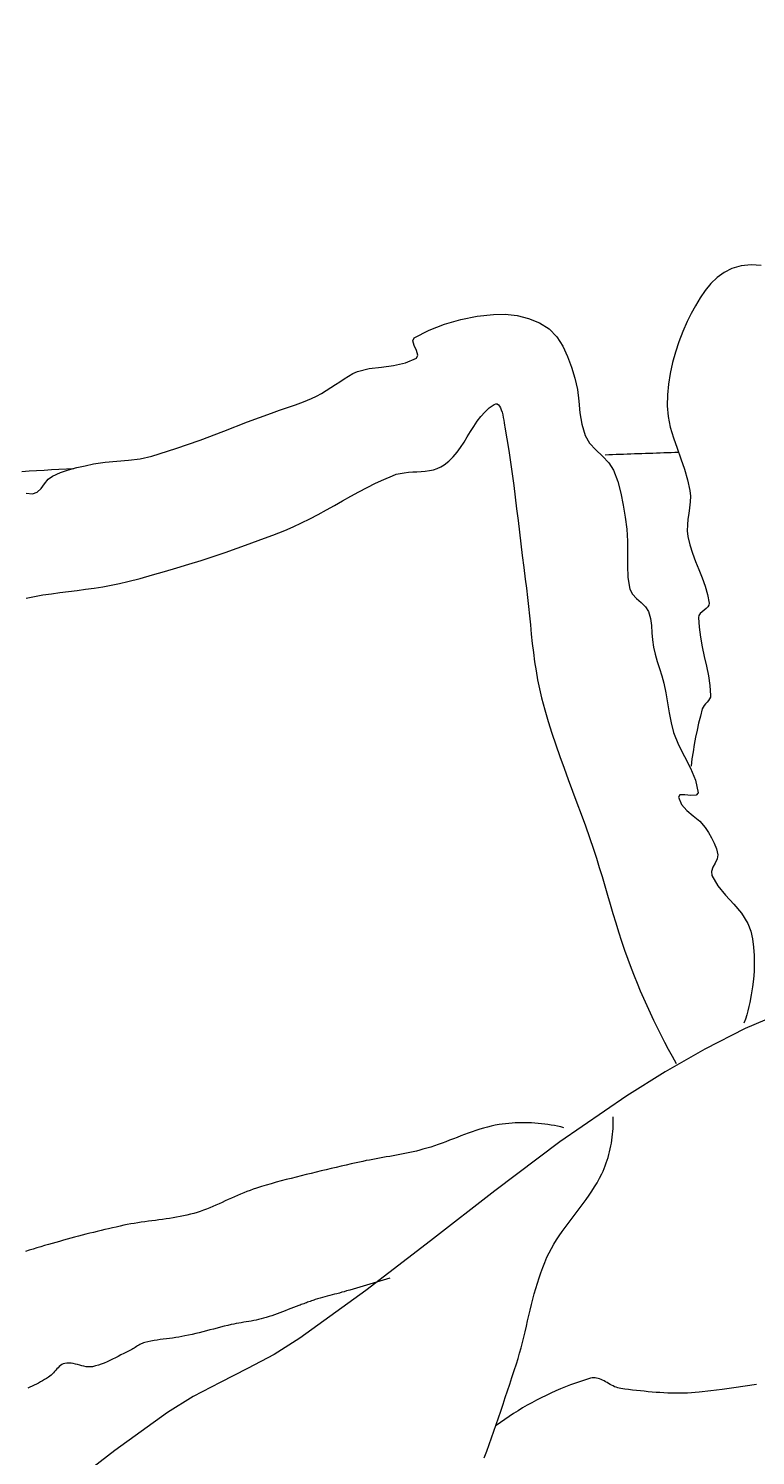
# Model space of a CAD drawing. Units: inches. Extents: x 1770 to 2988, y 1161 to 3221.
# Tile 27 of 44: x 2543 to 2562, y 2330 to 2368. Entities that reach past the tile are written whole.
import ezdxf

# ---------------------------------------------------------------- set-up
doc = ezdxf.new("R2010")
doc.units = ezdxf.units.IN
doc.layers.add('A-ANNO-DIMS', color=2, linetype='Continuous', lineweight=18)
doc.layers.add('A-FURN', color=8, linetype='Continuous', lineweight=13)
doc.styles.get("Standard").update_dxf_attribs({"font": 'arial.ttf'})
doc.dimstyles.get("Standard").update_dxf_attribs({"dimtxt": 0.18, "dimasz": 0.18, "dimexe": 0.18, "dimexo": 0.0625, "dimgap": 0.09, "dimtad": 0, "dimtih": 1, "dimtoh": 1, "dimdec": 4, "dimzin": 0, "dimdsep": 46, "dimtxsty": 'Standard', "dimcen": 0.09, "dimadec": 0, "dimazin": 0, "dimtfac": 1, "dimtdec": 4, "dimtofl": 0, "dimtmove": 0, "dimatfit": 3, "dimfxl": 1, "dimtolj": 1, "dimtzin": 0, "dimarcsym": 0})

# ---------------------------------------------------------------- blocks, each defined once
blk = doc.blocks.new('BED-DOUBLE-PLAN')
for p, q in [((35.584, 105.525), (35.385, 105.421)), ((35.831, 105.596), (35.584, 105.525)), ((36.086, 105.618), (35.831, 105.596)), ((36.348, 105.604), (36.086, 105.618)), ((35.039, 105.128), (34.89, 104.949)), ((35.203, 105.287), (35.039, 105.128)), ((35.385, 105.421), (35.203, 105.287)), ((34.755, 104.754), (34.633, 104.551)), ((34.89, 104.949), (34.755, 104.754)), ((34.633, 104.551), (34.523, 104.343)), ((27.681, 103.909), (28.087, 104.068)), ((28.087, 104.068), (28.506, 104.19)), ((28.506, 104.19), (28.933, 104.274)), ((28.933, 104.274), (29.364, 104.322)), ((29.364, 104.322), (29.669, 104.325)), ((29.669, 104.325), (29.977, 104.292)), ((29.977, 104.292), (30.279, 104.22)), ((30.279, 104.22), (30.562, 104.105)), ((30.562, 104.105), (30.817, 103.944)), ((34.422, 104.135), (34.307, 103.876)), ((34.523, 104.343), (34.422, 104.135)), ((27.256, 103.634), (27.295, 103.714)), ((27.291, 103.514), (27.256, 103.634)), ((27.295, 103.714), (27.681, 103.909)), ((30.817, 103.944), (31.018, 103.741)), ((31.018, 103.741), (31.173, 103.496)), ((34.203, 103.61), (34.112, 103.338)), ((34.307, 103.876), (34.203, 103.61)), ((27.352, 103.382), (27.291, 103.514)), ((27.349, 103.179), (27.388, 103.262)), ((27.388, 103.262), (27.352, 103.382)), ((31.173, 103.496), (31.294, 103.225)), ((34.112, 103.338), (34.035, 103.063)), ((25.811, 102.832), (26.119, 102.906)), ((26.119, 102.906), (26.438, 102.948)), ((26.438, 102.948), (26.756, 102.988)), ((26.756, 102.988), (27.064, 103.056)), ((27.064, 103.056), (27.349, 103.179)), ((31.294, 103.225), (31.395, 102.942)), ((31.395, 102.942), (31.487, 102.661)), ((34.035, 103.063), (33.974, 102.783)), ((25.242, 102.489), (25.354, 102.561)), ((25.354, 102.561), (25.464, 102.639)), ((25.464, 102.639), (25.574, 102.714)), ((25.574, 102.714), (25.689, 102.781)), ((25.689, 102.781), (25.811, 102.832)), ((31.487, 102.661), (31.558, 102.366)), ((33.93, 102.502), (33.904, 102.219)), ((33.974, 102.783), (33.93, 102.502)), ((24.406, 102.038), (24.611, 102.123)), ((24.611, 102.123), (24.742, 102.187)), ((24.742, 102.187), (24.869, 102.258)), ((24.869, 102.258), (24.993, 102.335)), ((24.993, 102.335), (25.117, 102.412)), ((25.117, 102.412), (25.242, 102.489)), ((31.558, 102.366), (31.593, 102.061)), ((33.904, 102.219), (33.898, 101.936)), ((22.945, 101.514), (23.568, 101.747)), ((23.568, 101.747), (23.778, 101.819)), ((23.778, 101.819), (23.988, 101.89)), ((23.988, 101.89), (24.198, 101.962)), ((24.198, 101.962), (24.406, 102.038)), ((29.035, 101.657), (29.139, 101.774)), ((29.139, 101.774), (29.253, 101.879)), ((29.253, 101.879), (29.38, 101.971)), ((29.38, 101.971), (29.42, 101.987)), ((29.42, 101.987), (29.457, 101.984)), ((29.457, 101.984), (29.489, 101.964)), ((29.489, 101.964), (29.518, 101.93)), ((29.518, 101.93), (29.543, 101.885)), ((29.543, 101.885), (29.566, 101.829)), ((29.566, 101.829), (29.586, 101.767)), ((29.586, 101.767), (29.603, 101.7)), ((31.593, 102.061), (31.62, 101.753)), ((31.62, 101.753), (31.664, 101.452)), ((33.898, 101.936), (33.922, 101.653)), ((22.324, 101.275), (22.945, 101.514)), ((28.763, 101.262), (28.85, 101.399)), ((28.85, 101.399), (28.939, 101.531)), ((28.939, 101.531), (29.035, 101.657)), ((29.603, 101.7), (29.618, 101.631)), ((29.618, 101.631), (29.631, 101.561)), ((29.631, 101.561), (29.643, 101.495)), ((29.643, 101.495), (29.653, 101.433)), ((29.653, 101.433), (29.662, 101.379)), ((29.662, 101.379), (29.714, 101.076)), ((31.664, 101.452), (31.751, 101.162)), ((33.922, 101.653), (33.978, 101.374)), ((33.978, 101.374), (34.058, 101.099)), ((21.074, 100.817), (21.701, 101.039)), ((21.701, 101.039), (22.324, 101.275)), ((28.593, 100.985), (28.679, 101.123)), ((28.679, 101.123), (28.763, 101.262)), ((29.714, 101.076), (29.763, 100.772)), ((31.751, 101.162), (31.871, 100.963)), ((34.058, 101.099), (34.153, 100.826)), ((20.44, 100.618), (21.074, 100.817)), ((28.31, 100.6), (28.411, 100.721)), ((28.411, 100.721), (28.505, 100.85)), ((28.505, 100.85), (28.593, 100.985)), ((29.763, 100.772), (29.808, 100.467)), ((31.871, 100.963), (32.032, 100.788)), ((32.032, 100.788), (32.208, 100.623)), ((32.279, 100.659), (32.375, 100.663)), ((32.375, 100.663), (32.47, 100.666)), ((32.47, 100.666), (32.566, 100.669)), ((32.566, 100.669), (32.662, 100.673)), ((32.662, 100.673), (32.758, 100.676)), ((32.758, 100.676), (32.854, 100.679)), ((32.854, 100.679), (32.949, 100.683)), ((32.949, 100.683), (33.045, 100.686)), ((33.045, 100.686), (33.141, 100.689)), ((33.141, 100.689), (33.237, 100.693)), ((33.237, 100.693), (33.333, 100.696)), ((33.333, 100.696), (33.429, 100.7)), ((33.429, 100.7), (33.524, 100.703)), ((33.524, 100.703), (33.62, 100.706)), ((33.62, 100.706), (33.716, 100.71)), ((33.716, 100.71), (33.812, 100.713)), ((33.812, 100.713), (33.908, 100.716)), ((33.908, 100.716), (34.004, 100.72)), ((34.004, 100.72), (34.099, 100.723)), ((34.099, 100.723), (34.195, 100.726)), ((34.153, 100.826), (34.252, 100.553)), ((17.437, 100.246), (17.631, 100.257)), ((17.631, 100.257), (17.825, 100.268)), ((17.825, 100.268), (18.018, 100.279)), ((18.018, 100.279), (18.212, 100.29)), ((18.057, 100.19), (18.267, 100.262)), ((18.212, 100.29), (18.406, 100.301)), ((18.267, 100.262), (18.482, 100.321)), ((18.482, 100.321), (18.7, 100.371)), ((18.7, 100.371), (18.918, 100.416)), ((18.918, 100.416), (19.222, 100.462)), ((19.222, 100.462), (19.529, 100.49)), ((19.529, 100.49), (19.836, 100.515)), ((19.836, 100.515), (20.141, 100.553)), ((20.141, 100.553), (20.44, 100.618)), ((27.688, 100.246), (27.792, 100.267)), ((27.792, 100.267), (27.892, 100.297)), ((27.892, 100.297), (27.987, 100.338)), ((27.987, 100.338), (28.077, 100.392)), ((28.077, 100.392), (28.2, 100.489)), ((28.2, 100.489), (28.31, 100.6)), ((29.808, 100.467), (29.85, 100.162)), ((32.208, 100.623), (32.371, 100.449)), ((32.371, 100.449), (32.495, 100.252)), ((34.252, 100.553), (34.347, 100.28)), ((34.347, 100.28), (34.429, 100.003)), ((17.05, 100.224), (17.244, 100.235)), ((17.244, 100.235), (17.437, 100.246)), ((17.553, 99.78), (17.645, 99.9)), ((17.645, 99.9), (17.741, 100.016)), ((17.741, 100.016), (17.853, 100.102)), ((17.853, 100.102), (18.057, 100.19)), ((26.064, 99.803), (26.281, 99.912)), ((26.281, 99.912), (26.5, 100.015)), ((26.5, 100.015), (26.723, 100.111)), ((26.723, 100.111), (26.823, 100.146)), ((26.823, 100.146), (26.927, 100.171)), ((26.927, 100.171), (27.034, 100.188)), ((27.034, 100.188), (27.143, 100.2)), ((27.143, 100.2), (27.253, 100.208)), ((27.253, 100.208), (27.363, 100.215)), ((27.363, 100.215), (27.473, 100.222)), ((27.473, 100.222), (27.582, 100.232)), ((27.582, 100.232), (27.688, 100.246)), ((29.85, 100.162), (29.89, 99.857)), ((32.495, 100.252), (32.606, 99.957)), ((32.606, 99.957), (32.689, 99.653)), ((34.429, 100.003), (34.488, 99.723)), ((17.16, 99.657), (17.329, 99.635)), ((17.329, 99.635), (17.452, 99.683)), ((17.452, 99.683), (17.553, 99.78)), ((25.424, 99.453), (25.636, 99.572)), ((25.636, 99.572), (25.85, 99.689)), ((25.85, 99.689), (26.064, 99.803)), ((29.89, 99.857), (29.929, 99.551)), ((29.929, 99.551), (29.966, 99.246)), ((32.689, 99.653), (32.75, 99.342)), ((34.488, 99.723), (34.501, 99.574)), ((34.501, 99.574), (34.496, 99.425)), ((24.786, 99.099), (25, 99.215)), ((25, 99.215), (25.212, 99.334)), ((25.212, 99.334), (25.424, 99.453)), ((29.966, 99.246), (30.003, 98.94)), ((32.75, 99.342), (32.799, 99.027)), ((34.48, 99.274), (34.459, 99.124)), ((34.496, 99.425), (34.48, 99.274)), ((23.911, 98.681), (24.134, 98.776)), ((24.134, 98.776), (24.354, 98.878)), ((24.354, 98.878), (24.571, 98.986)), ((24.571, 98.986), (24.786, 99.099)), ((30.003, 98.94), (30.039, 98.634)), ((32.799, 99.027), (32.842, 98.713)), ((34.423, 98.823), (34.42, 98.674)), ((34.438, 98.973), (34.423, 98.823)), ((34.459, 99.124), (34.438, 98.973)), ((22.983, 98.327), (23.293, 98.442)), ((23.293, 98.442), (23.603, 98.56)), ((23.603, 98.56), (23.911, 98.681)), ((30.039, 98.634), (30.076, 98.328)), ((32.842, 98.713), (32.864, 98.4)), ((32.864, 98.4), (32.862, 98.084)), ((34.42, 98.674), (34.435, 98.525)), ((34.435, 98.525), (34.485, 98.303)), ((22.043, 98), (22.358, 98.106)), ((22.358, 98.106), (22.671, 98.215)), ((22.671, 98.215), (22.983, 98.327)), ((30.076, 98.328), (30.113, 98.022)), ((30.113, 98.022), (30.152, 97.716)), ((32.862, 98.084), (32.856, 97.768)), ((34.485, 98.303), (34.554, 98.085)), ((34.554, 98.085), (34.635, 97.87)), ((20.777, 97.608), (21.095, 97.702)), ((21.095, 97.702), (21.412, 97.798)), ((21.412, 97.798), (21.728, 97.898)), ((21.728, 97.898), (22.043, 98)), ((30.152, 97.716), (30.192, 97.411)), ((32.856, 97.768), (32.868, 97.455)), ((34.635, 97.87), (34.722, 97.657)), ((34.722, 97.657), (34.808, 97.443)), ((19.381, 97.247), (19.6, 97.292)), ((19.6, 97.292), (19.818, 97.344)), ((19.818, 97.344), (20.138, 97.429)), ((20.138, 97.429), (20.458, 97.517)), ((20.458, 97.517), (20.777, 97.608)), ((30.192, 97.411), (30.222, 97.172)), ((32.868, 97.455), (32.921, 97.148)), ((34.808, 97.443), (34.886, 97.228)), ((17.161, 96.913), (17.38, 96.957)), ((17.38, 96.957), (17.602, 96.995)), ((17.602, 96.995), (17.824, 97.028)), ((17.824, 97.028), (18.046, 97.058)), ((18.046, 97.058), (18.269, 97.086)), ((18.269, 97.086), (18.493, 97.114)), ((18.493, 97.114), (18.716, 97.143)), ((18.716, 97.143), (18.938, 97.174)), ((18.938, 97.174), (19.16, 97.208)), ((19.16, 97.208), (19.381, 97.247)), ((30.222, 97.172), (30.25, 96.932)), ((30.25, 96.932), (30.275, 96.692)), ((32.921, 97.148), (32.988, 97.015)), ((32.988, 97.015), (33.094, 96.903)), ((33.094, 96.903), (33.215, 96.799)), ((34.886, 97.228), (34.95, 97.009)), ((34.95, 97.009), (34.993, 96.785)), ((30.275, 96.692), (30.3, 96.452)), ((33.215, 96.799), (33.328, 96.689)), ((33.328, 96.689), (33.41, 96.561)), ((33.41, 96.561), (33.462, 96.384)), ((34.806, 96.555), (34.759, 96.511)), ((34.86, 96.597), (34.806, 96.555)), ((34.912, 96.639), (34.86, 96.597)), ((34.957, 96.683), (34.912, 96.639)), ((34.986, 96.731), (34.957, 96.683)), ((34.993, 96.785), (34.986, 96.731)), ((30.3, 96.452), (30.324, 96.211)), ((30.324, 96.211), (30.349, 95.971)), ((33.462, 96.384), (33.486, 96.199)), ((33.486, 96.199), (33.497, 96.01)), ((34.725, 96.462), (34.713, 96.407)), ((34.713, 96.407), (34.729, 96.151)), ((34.759, 96.511), (34.725, 96.462)), ((30.349, 95.971), (30.375, 95.731)), ((33.497, 96.01), (33.509, 95.822)), ((33.509, 95.822), (33.535, 95.636)), ((34.729, 96.151), (34.763, 95.896)), ((34.763, 95.896), (34.811, 95.643)), ((30.375, 95.731), (30.404, 95.491)), ((30.404, 95.491), (30.436, 95.252)), ((33.535, 95.636), (33.582, 95.446)), ((33.582, 95.446), (33.638, 95.258)), ((34.811, 95.643), (34.865, 95.39)), ((30.436, 95.252), (30.473, 95.014)), ((33.638, 95.258), (33.698, 95.071)), ((33.698, 95.071), (33.755, 94.883)), ((34.865, 95.39), (34.921, 95.137)), ((34.921, 95.137), (34.971, 94.884)), ((30.473, 95.014), (30.515, 94.777)), ((30.515, 94.777), (30.563, 94.541)), ((33.755, 94.883), (33.806, 94.694)), ((33.806, 94.694), (33.859, 94.435)), ((34.971, 94.884), (35.009, 94.629)), ((30.563, 94.541), (30.618, 94.307)), ((30.618, 94.307), (30.701, 93.997)), ((33.859, 94.435), (33.903, 94.175)), ((35.024, 94.323), (35.004, 94.278)), ((35.009, 94.629), (35.031, 94.373)), ((35.031, 94.373), (35.024, 94.323)), ((30.701, 93.997), (30.791, 93.689)), ((33.903, 94.175), (33.946, 93.914)), ((34.812, 94.017), (34.763, 93.833)), ((34.833, 94.065), (34.812, 94.017)), ((34.863, 94.11), (34.833, 94.065)), ((34.899, 94.152), (34.863, 94.11)), ((34.938, 94.193), (34.899, 94.152)), ((34.974, 94.235), (34.938, 94.193)), ((35.004, 94.278), (34.974, 94.235)), ((30.791, 93.689), (30.887, 93.383)), ((33.946, 93.914), (33.997, 93.655)), ((33.997, 93.655), (34.064, 93.401)), ((34.718, 93.649), (34.676, 93.463)), ((34.763, 93.833), (34.718, 93.649)), ((30.887, 93.383), (30.989, 93.078)), ((34.064, 93.401), (34.191, 93.084)), ((34.637, 93.277), (34.602, 93.089)), ((34.676, 93.463), (34.637, 93.277)), ((30.989, 93.078), (31.095, 92.775)), ((34.191, 93.084), (34.349, 92.776)), ((34.571, 92.902), (34.543, 92.713)), ((34.602, 93.089), (34.571, 92.902)), ((31.095, 92.775), (31.204, 92.473)), ((31.204, 92.473), (31.315, 92.172)), ((34.349, 92.776), (34.507, 92.47)), ((34.507, 92.47), (34.635, 92.156)), ((34.543, 92.713), (34.519, 92.525)), ((31.315, 92.172), (31.427, 91.87)), ((34.635, 92.156), (34.701, 91.828)), ((31.427, 91.87), (31.54, 91.569)), ((34.229, 91.774), (34.188, 91.712)), ((34.188, 91.712), (34.269, 91.526)), ((34.357, 91.777), (34.229, 91.774)), ((34.516, 91.761), (34.357, 91.777)), ((34.649, 91.765), (34.516, 91.761)), ((34.701, 91.828), (34.649, 91.765)), ((31.54, 91.569), (31.652, 91.268)), ((34.269, 91.526), (34.408, 91.37)), ((34.408, 91.37), (34.576, 91.228)), ((31.652, 91.268), (31.762, 90.966)), ((31.762, 90.966), (31.869, 90.663)), ((34.576, 91.228), (34.746, 91.085)), ((34.746, 91.085), (34.888, 90.925)), ((31.869, 90.663), (31.973, 90.359)), ((34.888, 90.925), (34.975, 90.793)), ((34.975, 90.793), (35.056, 90.655)), ((35.056, 90.655), (35.126, 90.512)), ((31.973, 90.359), (32.05, 90.12)), ((35.126, 90.512), (35.181, 90.364)), ((35.181, 90.364), (35.215, 90.211)), ((35.215, 90.211), (35.201, 90.1)), ((32.05, 90.12), (32.125, 89.88)), ((32.125, 89.88), (32.197, 89.64)), ((35.091, 89.882), (35.052, 89.775)), ((35.151, 89.99), (35.091, 89.882)), ((35.201, 90.1), (35.151, 89.99)), ((32.197, 89.64), (32.269, 89.399)), ((35.052, 89.775), (35.063, 89.671)), ((35.063, 89.671), (35.219, 89.402)), ((32.269, 89.399), (32.34, 89.158)), ((32.34, 89.158), (32.41, 88.917)), ((35.219, 89.402), (35.418, 89.158)), ((35.418, 89.158), (35.633, 88.923)), ((32.41, 88.917), (32.481, 88.676)), ((35.633, 88.923), (35.836, 88.68)), ((32.481, 88.676), (32.554, 88.436)), ((32.554, 88.436), (32.628, 88.196)), ((35.836, 88.68), (36.001, 88.415)), ((36.001, 88.415), (36.077, 88.217)), ((32.628, 88.196), (32.705, 87.957)), ((32.705, 87.957), (32.785, 87.719)), ((36.077, 88.217), (36.124, 88.01)), ((36.124, 88.01), (36.151, 87.797)), ((32.785, 87.719), (32.868, 87.483)), ((36.151, 87.797), (36.164, 87.581)), ((32.868, 87.483), (32.956, 87.248)), ((32.956, 87.248), (33.033, 87.051)), ((36.164, 87.581), (36.171, 87.367)), ((36.171, 87.367), (36.167, 87.163)), ((33.033, 87.051), (33.113, 86.854)), ((33.113, 86.854), (33.194, 86.659)), ((36.149, 86.96), (36.121, 86.757)), ((36.167, 87.163), (36.149, 86.96)), ((33.194, 86.659), (33.278, 86.464)), ((36.087, 86.555), (36.051, 86.354)), ((36.121, 86.757), (36.087, 86.555)), ((33.278, 86.464), (33.364, 86.271)), ((33.364, 86.271), (33.453, 86.078)), ((37.023, 86.135), (35.936, 85.668)), ((36.003, 86.134), (35.973, 86.026)), ((36.029, 86.243), (36.003, 86.134)), ((36.051, 86.354), (36.029, 86.243)), ((33.453, 86.078), (33.543, 85.886)), ((33.543, 85.886), (33.636, 85.696)), ((35.938, 85.919), (35.899, 85.813)), ((35.973, 86.026), (35.938, 85.919)), ((33.636, 85.696), (33.73, 85.506)), ((33.73, 85.506), (33.827, 85.318)), ((35.936, 85.668), (34.877, 85.131)), ((33.827, 85.318), (33.926, 85.131)), ((34.877, 85.131), (33.846, 84.541)), ((33.926, 85.131), (34.027, 84.945)), ((34.027, 84.945), (34.13, 84.76)), ((33.846, 84.541), (32.841, 83.914)), ((32.841, 83.914), (31.092, 82.71)), ((29.303, 83.123), (29.202, 83.099)), ((29.405, 83.144), (29.303, 83.123)), ((29.508, 83.162), (29.405, 83.144)), ((29.592, 83.174), (29.508, 83.162)), ((29.676, 83.184), (29.592, 83.174)), ((29.761, 83.193), (29.676, 83.184)), ((29.846, 83.2), (29.761, 83.193)), ((29.931, 83.205), (29.846, 83.2)), ((30.016, 83.208), (29.931, 83.205)), ((30.102, 83.21), (30.016, 83.208)), ((30.187, 83.21), (30.102, 83.21)), ((30.273, 83.209), (30.187, 83.21)), ((30.358, 83.205), (30.273, 83.209)), ((30.444, 83.2), (30.358, 83.205)), ((30.529, 83.194), (30.444, 83.2)), ((30.614, 83.185), (30.529, 83.194)), ((30.699, 83.175), (30.614, 83.185)), ((30.784, 83.163), (30.699, 83.175)), ((30.868, 83.15), (30.784, 83.163)), ((30.952, 83.135), (30.868, 83.15)), ((31.036, 83.118), (30.952, 83.135)), ((31.119, 83.1), (31.036, 83.118)), ((32.486, 83.292), (32.483, 83.369)), ((32.483, 83.063), (32.486, 83.14)), ((32.487, 83.216), (32.486, 83.292)), ((32.486, 83.14), (32.487, 83.216)), ((28.216, 82.752), (28.118, 82.715)), ((28.314, 82.79), (28.216, 82.752)), ((28.411, 82.829), (28.314, 82.79)), ((28.509, 82.867), (28.411, 82.829)), ((28.607, 82.904), (28.509, 82.867)), ((28.705, 82.941), (28.607, 82.904)), ((28.804, 82.976), (28.705, 82.941)), ((28.902, 83.01), (28.804, 82.976)), ((29.002, 83.042), (28.902, 83.01)), ((29.102, 83.072), (29.002, 83.042)), ((29.202, 83.099), (29.102, 83.072)), ((31.201, 83.08), (31.119, 83.1)), ((32.441, 82.68), (32.453, 82.757)), ((32.453, 82.757), (32.463, 82.833)), ((32.463, 82.833), (32.472, 82.91)), ((32.472, 82.91), (32.478, 82.986)), ((32.478, 82.986), (32.483, 83.063)), ((26.915, 82.381), (26.827, 82.364)), ((27.002, 82.397), (26.915, 82.381)), ((27.089, 82.415), (27.002, 82.397)), ((27.176, 82.433), (27.089, 82.415)), ((27.263, 82.452), (27.176, 82.433)), ((27.35, 82.472), (27.263, 82.452)), ((27.436, 82.493), (27.35, 82.472)), ((27.522, 82.516), (27.436, 82.493)), ((27.623, 82.544), (27.522, 82.516)), ((27.723, 82.574), (27.623, 82.544)), ((27.822, 82.607), (27.723, 82.574)), ((27.921, 82.642), (27.822, 82.607)), ((28.02, 82.678), (27.921, 82.642)), ((28.118, 82.715), (28.02, 82.678)), ((31.092, 82.71), (29.393, 81.433)), ((32.353, 82.305), (32.374, 82.379)), ((32.374, 82.379), (32.393, 82.454)), ((32.393, 82.454), (32.411, 82.529)), ((32.411, 82.529), (32.427, 82.605)), ((32.427, 82.605), (32.441, 82.68)), ((25.123, 82.012), (24.992, 81.981)), ((25.254, 82.042), (25.123, 82.012)), ((25.385, 82.073), (25.254, 82.042)), ((25.516, 82.103), (25.385, 82.073)), ((25.647, 82.133), (25.516, 82.103)), ((25.778, 82.164), (25.647, 82.133)), ((25.865, 82.183), (25.778, 82.164)), ((25.952, 82.202), (25.865, 82.183)), ((26.039, 82.22), (25.952, 82.202)), ((26.126, 82.237), (26.039, 82.22)), ((26.214, 82.254), (26.126, 82.237)), ((26.301, 82.27), (26.214, 82.254)), ((26.389, 82.286), (26.301, 82.27)), ((26.477, 82.301), (26.389, 82.286)), ((26.564, 82.317), (26.477, 82.301)), ((26.652, 82.333), (26.564, 82.317)), ((26.74, 82.348), (26.652, 82.333)), ((26.827, 82.364), (26.74, 82.348)), ((32.221, 81.946), (32.251, 82.016)), ((32.251, 82.016), (32.279, 82.087)), ((32.279, 82.087), (32.305, 82.159)), ((32.305, 82.159), (32.33, 82.232)), ((32.33, 82.232), (32.353, 82.305)), ((23.69, 81.654), (23.56, 81.617)), ((23.819, 81.689), (23.69, 81.654)), ((23.949, 81.724), (23.819, 81.689)), ((24.079, 81.758), (23.949, 81.724)), ((24.209, 81.791), (24.079, 81.758)), ((24.339, 81.824), (24.209, 81.791)), ((24.47, 81.856), (24.339, 81.824)), ((24.6, 81.888), (24.47, 81.856)), ((24.731, 81.92), (24.6, 81.888)), ((24.862, 81.951), (24.731, 81.92)), ((24.992, 81.981), (24.862, 81.951)), ((32.003, 81.534), (32.069, 81.645)), ((32.069, 81.645), (32.132, 81.76)), ((32.132, 81.76), (32.189, 81.876)), ((32.189, 81.876), (32.221, 81.946)), ((22.6, 81.277), (22.52, 81.24)), ((22.681, 81.313), (22.6, 81.277)), ((22.762, 81.348), (22.681, 81.313)), ((22.843, 81.382), (22.762, 81.348)), ((22.925, 81.414), (22.843, 81.382)), ((23.008, 81.445), (22.925, 81.414)), ((23.091, 81.475), (23.008, 81.445)), ((23.174, 81.502), (23.091, 81.475)), ((23.303, 81.541), (23.174, 81.502)), ((23.431, 81.58), (23.303, 81.541)), ((23.56, 81.617), (23.431, 81.58)), ((29.393, 81.433), (27.716, 80.125)), ((31.784, 81.208), (31.86, 81.315)), ((31.86, 81.315), (31.933, 81.424)), ((31.933, 81.424), (32.003, 81.534)), ((21.708, 80.896), (21.625, 80.868)), ((21.791, 80.925), (21.708, 80.896)), ((21.873, 80.956), (21.791, 80.925)), ((21.955, 80.989), (21.873, 80.956)), ((22.037, 81.023), (21.955, 80.989)), ((22.118, 81.058), (22.037, 81.023)), ((22.198, 81.094), (22.118, 81.058)), ((22.279, 81.13), (22.198, 81.094)), ((22.359, 81.167), (22.279, 81.13)), ((22.439, 81.204), (22.359, 81.167)), ((22.52, 81.24), (22.439, 81.204)), ((31.468, 80.789), (31.548, 80.893)), ((31.548, 80.893), (31.628, 80.997)), ((31.628, 80.997), (31.707, 81.102)), ((31.707, 81.102), (31.784, 81.208)), ((19.613, 80.509), (19.514, 80.487)), ((19.712, 80.531), (19.613, 80.509)), ((19.803, 80.549), (19.712, 80.531)), ((19.894, 80.567), (19.803, 80.549)), ((19.985, 80.582), (19.894, 80.567)), ((20.077, 80.597), (19.985, 80.582)), ((20.169, 80.611), (20.077, 80.597)), ((20.261, 80.624), (20.169, 80.611)), ((20.353, 80.637), (20.261, 80.624)), ((20.445, 80.649), (20.353, 80.637)), ((20.537, 80.661), (20.445, 80.649)), ((20.63, 80.673), (20.537, 80.661)), ((20.722, 80.686), (20.63, 80.673)), ((20.814, 80.699), (20.722, 80.686)), ((20.905, 80.712), (20.814, 80.699)), ((20.997, 80.727), (20.905, 80.712)), ((21.088, 80.742), (20.997, 80.727)), ((21.18, 80.759), (21.088, 80.742)), ((21.27, 80.778), (21.18, 80.759)), ((21.361, 80.798), (21.27, 80.778)), ((21.451, 80.819), (21.361, 80.798)), ((21.54, 80.843), (21.451, 80.819)), ((21.625, 80.868), (21.54, 80.843)), ((31.231, 80.474), (31.309, 80.58)), ((31.309, 80.58), (31.388, 80.684)), ((31.388, 80.684), (31.468, 80.789)), ((18.135, 80.14), (18.037, 80.113)), ((18.233, 80.167), (18.135, 80.14)), ((18.331, 80.194), (18.233, 80.167)), ((18.429, 80.22), (18.331, 80.194)), ((18.527, 80.246), (18.429, 80.22)), ((18.625, 80.272), (18.527, 80.246)), ((18.724, 80.298), (18.625, 80.272)), ((18.822, 80.323), (18.724, 80.298)), ((18.921, 80.347), (18.822, 80.323)), ((19.019, 80.372), (18.921, 80.347)), ((19.118, 80.395), (19.019, 80.372)), ((19.217, 80.419), (19.118, 80.395)), ((19.316, 80.442), (19.217, 80.419)), ((19.415, 80.465), (19.316, 80.442)), ((19.514, 80.487), (19.415, 80.465)), ((30.939, 80.041), (31.008, 80.152)), ((31.008, 80.152), (31.079, 80.261)), ((31.079, 80.261), (31.154, 80.368)), ((31.154, 80.368), (31.231, 80.474)), ((17.245, 79.878), (17.145, 79.846)), ((17.344, 79.909), (17.245, 79.878)), ((17.444, 79.94), (17.344, 79.909)), ((17.544, 79.97), (17.444, 79.94)), ((17.644, 80), (17.544, 79.97)), ((17.744, 80.029), (17.644, 80)), ((17.842, 80.057), (17.744, 80.029)), ((17.939, 80.085), (17.842, 80.057)), ((18.037, 80.113), (17.939, 80.085)), ((27.716, 80.125), (26.032, 78.826)), ((30.757, 79.696), (30.813, 79.814)), ((30.813, 79.814), (30.874, 79.929)), ((30.874, 79.929), (30.939, 80.041)), ((30.597, 79.294), (30.647, 79.429)), ((30.647, 79.429), (30.7, 79.563)), ((30.7, 79.563), (30.757, 79.696)), ((26.223, 79.021), (26.136, 78.995)), ((26.31, 79.047), (26.223, 79.021)), ((26.396, 79.073), (26.31, 79.047)), ((26.483, 79.1), (26.396, 79.073)), ((26.569, 79.126), (26.483, 79.1)), ((26.656, 79.153), (26.569, 79.126)), ((30.467, 78.88), (30.508, 79.019)), ((30.508, 79.019), (30.551, 79.157)), ((30.551, 79.157), (30.597, 79.294)), ((26.032, 78.826), (24.311, 77.58)), ((24.898, 78.645), (24.835, 78.627)), ((24.961, 78.662), (24.898, 78.645)), ((25.024, 78.679), (24.961, 78.662)), ((25.087, 78.696), (25.024, 78.679)), ((25.151, 78.713), (25.087, 78.696)), ((25.214, 78.73), (25.151, 78.713)), ((25.277, 78.746), (25.214, 78.73)), ((25.34, 78.763), (25.277, 78.746)), ((25.403, 78.781), (25.34, 78.763)), ((25.466, 78.798), (25.403, 78.781)), ((25.529, 78.816), (25.466, 78.798)), ((25.616, 78.841), (25.529, 78.816)), ((25.703, 78.867), (25.616, 78.841)), ((25.79, 78.892), (25.703, 78.867)), ((25.876, 78.918), (25.79, 78.892)), ((25.963, 78.943), (25.876, 78.918)), ((26.05, 78.969), (25.963, 78.943)), ((26.136, 78.995), (26.05, 78.969)), ((30.391, 78.601), (30.428, 78.741)), ((30.428, 78.741), (30.467, 78.88)), ((23.858, 78.274), (23.788, 78.247)), ((23.928, 78.301), (23.858, 78.274)), ((23.999, 78.329), (23.928, 78.301)), ((24.069, 78.356), (23.999, 78.329)), ((24.139, 78.383), (24.069, 78.356)), ((24.21, 78.409), (24.139, 78.383)), ((24.28, 78.435), (24.21, 78.409)), ((24.313, 78.447), (24.28, 78.435)), ((24.346, 78.459), (24.313, 78.447)), ((24.379, 78.472), (24.346, 78.459)), ((24.412, 78.484), (24.379, 78.472)), ((24.445, 78.497), (24.412, 78.484)), ((24.478, 78.509), (24.445, 78.497)), ((24.511, 78.521), (24.478, 78.509)), ((24.544, 78.533), (24.511, 78.521)), ((24.577, 78.545), (24.544, 78.533)), ((24.61, 78.557), (24.577, 78.545)), ((24.643, 78.568), (24.61, 78.557)), ((24.676, 78.579), (24.643, 78.568)), ((24.71, 78.59), (24.676, 78.579)), ((24.772, 78.609), (24.71, 78.59)), ((24.835, 78.627), (24.772, 78.609)), ((30.288, 78.177), (30.321, 78.319)), ((30.321, 78.319), (30.356, 78.46)), ((30.356, 78.46), (30.391, 78.601)), ((22.332, 77.894), (22.239, 77.871)), ((22.425, 77.917), (22.332, 77.894)), ((22.518, 77.938), (22.425, 77.917)), ((22.583, 77.952), (22.518, 77.938)), ((22.648, 77.965), (22.583, 77.952)), ((22.713, 77.977), (22.648, 77.965)), ((22.778, 77.988), (22.713, 77.977)), ((22.843, 77.999), (22.778, 77.988)), ((22.908, 78.01), (22.843, 77.999)), ((22.973, 78.021), (22.908, 78.01)), ((23.038, 78.032), (22.973, 78.021)), ((23.103, 78.044), (23.038, 78.032)), ((23.168, 78.057), (23.103, 78.044)), ((23.232, 78.071), (23.168, 78.057)), ((23.296, 78.086), (23.232, 78.071)), ((23.36, 78.103), (23.296, 78.086)), ((23.432, 78.124), (23.36, 78.103)), ((23.504, 78.147), (23.432, 78.124)), ((23.575, 78.171), (23.504, 78.147)), ((23.646, 78.195), (23.575, 78.171)), ((23.717, 78.221), (23.646, 78.195)), ((23.788, 78.247), (23.717, 78.221)), ((30.188, 77.753), (30.221, 77.894)), ((30.221, 77.894), (30.254, 78.036)), ((30.254, 78.036), (30.288, 78.177)), ((20.5, 77.522), (20.42, 77.507)), ((20.581, 77.535), (20.5, 77.522)), ((20.662, 77.547), (20.581, 77.535)), ((20.743, 77.558), (20.662, 77.547)), ((20.824, 77.568), (20.743, 77.558)), ((20.905, 77.578), (20.824, 77.568)), ((20.986, 77.588), (20.905, 77.578)), ((21.067, 77.599), (20.986, 77.588)), ((21.148, 77.612), (21.067, 77.599)), ((21.229, 77.625), (21.148, 77.612)), ((21.309, 77.641), (21.229, 77.625)), ((21.402, 77.661), (21.309, 77.641)), ((21.496, 77.682), (21.402, 77.661)), ((21.589, 77.704), (21.496, 77.682)), ((21.682, 77.727), (21.589, 77.704)), ((21.775, 77.751), (21.682, 77.727)), ((21.868, 77.775), (21.775, 77.751)), ((21.961, 77.799), (21.868, 77.775)), ((22.053, 77.823), (21.961, 77.799)), ((22.146, 77.847), (22.053, 77.823)), ((22.239, 77.871), (22.146, 77.847)), ((24.311, 77.58), (23.639, 77.161)), ((30.118, 77.47), (30.153, 77.611)), ((30.153, 77.611), (30.188, 77.753)), ((19.709, 77.184), (19.636, 77.147)), ((19.781, 77.22), (19.709, 77.184)), ((19.854, 77.255), (19.781, 77.22)), ((19.886, 77.27), (19.854, 77.255)), ((19.917, 77.287), (19.886, 77.27)), ((19.948, 77.305), (19.917, 77.287)), ((19.978, 77.324), (19.948, 77.305)), ((20.008, 77.343), (19.978, 77.324)), ((20.039, 77.363), (20.008, 77.343)), ((20.069, 77.382), (20.039, 77.363)), ((20.1, 77.4), (20.069, 77.382)), ((20.131, 77.417), (20.1, 77.4)), ((20.162, 77.433), (20.131, 77.417)), ((20.194, 77.448), (20.162, 77.433)), ((20.227, 77.46), (20.194, 77.448)), ((20.261, 77.471), (20.227, 77.46)), ((20.34, 77.49), (20.261, 77.471)), ((20.42, 77.507), (20.34, 77.49)), ((23.639, 77.161), (22.938, 76.788)), ((30.002, 77.051), (30.043, 77.19)), ((30.043, 77.19), (30.081, 77.33)), ((30.081, 77.33), (30.118, 77.47)), ((17.965, 76.781), (17.935, 76.747)), ((17.995, 76.813), (17.965, 76.781)), ((18.026, 76.843), (17.995, 76.813)), ((18.058, 76.87), (18.026, 76.843)), ((18.093, 76.893), (18.058, 76.87)), ((18.13, 76.912), (18.093, 76.893)), ((18.17, 76.925), (18.13, 76.912)), ((18.225, 76.934), (18.17, 76.925)), ((18.28, 76.935), (18.225, 76.934)), ((18.336, 76.931), (18.28, 76.935)), ((18.391, 76.921), (18.336, 76.931)), ((18.447, 76.909), (18.391, 76.921)), ((18.503, 76.894), (18.447, 76.909)), ((18.56, 76.878), (18.503, 76.894)), ((18.616, 76.863), (18.56, 76.878)), ((18.672, 76.849), (18.616, 76.863)), ((18.728, 76.839), (18.672, 76.849)), ((18.784, 76.833), (18.728, 76.839)), ((18.839, 76.832), (18.784, 76.833)), ((18.894, 76.839), (18.839, 76.832)), ((18.973, 76.857), (18.894, 76.839)), ((19.049, 76.879), (18.973, 76.857)), ((19.125, 76.905), (19.049, 76.879)), ((19.2, 76.934), (19.125, 76.905)), ((19.274, 76.966), (19.2, 76.934)), ((19.347, 77), (19.274, 76.966)), ((19.42, 77.035), (19.347, 77)), ((19.492, 77.072), (19.42, 77.035)), ((19.564, 77.109), (19.492, 77.072)), ((19.636, 77.147), (19.564, 77.109)), ((22.938, 76.788), (22.227, 76.429)), ((29.902, 76.736), (29.959, 76.913)), ((29.959, 76.913), (30.002, 77.051)), ((17.483, 76.408), (17.429, 76.38)), ((17.536, 76.439), (17.483, 76.408)), ((17.589, 76.469), (17.536, 76.439)), ((17.642, 76.501), (17.589, 76.469)), ((17.694, 76.532), (17.642, 76.501)), ((17.746, 76.564), (17.694, 76.532)), ((17.781, 76.588), (17.746, 76.564)), ((17.815, 76.616), (17.781, 76.588)), ((17.846, 76.647), (17.815, 76.616)), ((17.877, 76.679), (17.846, 76.647)), ((17.906, 76.713), (17.877, 76.679)), ((17.935, 76.747), (17.906, 76.713)), ((22.227, 76.429), (21.526, 76.056)), ((29.786, 76.384), (29.844, 76.56)), ((29.844, 76.56), (29.902, 76.736)), ((31.503, 76.409), (31.372, 76.361)), ((31.633, 76.454), (31.503, 76.409)), ((31.765, 76.497), (31.633, 76.454)), ((31.897, 76.537), (31.765, 76.497)), ((31.936, 76.546), (31.897, 76.537)), ((31.976, 76.55), (31.936, 76.546)), ((32.016, 76.549), (31.976, 76.55)), ((32.055, 76.543), (32.016, 76.549)), ((32.094, 76.533), (32.055, 76.543)), ((32.133, 76.521), (32.094, 76.533)), ((32.172, 76.505), (32.133, 76.521)), ((32.211, 76.487), (32.172, 76.505)), ((32.249, 76.467), (32.211, 76.487)), ((32.288, 76.445), (32.249, 76.467)), ((32.327, 76.423), (32.288, 76.445)), ((32.366, 76.401), (32.327, 76.423)), ((17.263, 76.303), (17.207, 76.282)), ((17.319, 76.326), (17.263, 76.303)), ((17.374, 76.352), (17.319, 76.326)), ((17.429, 76.38), (17.374, 76.352)), ((21.526, 76.056), (20.852, 75.639)), ((29.611, 75.856), (29.67, 76.032)), ((29.67, 76.032), (29.728, 76.208)), ((29.728, 76.208), (29.786, 76.384)), ((30.734, 76.088), (30.61, 76.027)), ((30.86, 76.147), (30.734, 76.088)), ((30.987, 76.204), (30.86, 76.147)), ((31.115, 76.259), (30.987, 76.204)), ((31.243, 76.311), (31.115, 76.259)), ((31.372, 76.361), (31.243, 76.311)), ((32.406, 76.378), (32.366, 76.401)), ((32.445, 76.356), (32.406, 76.378)), ((32.485, 76.336), (32.445, 76.356)), ((32.524, 76.317), (32.485, 76.336)), ((32.564, 76.3), (32.524, 76.317)), ((32.605, 76.286), (32.564, 76.3)), ((32.646, 76.275), (32.605, 76.286)), ((32.687, 76.268), (32.646, 76.275)), ((32.789, 76.255), (32.687, 76.268)), ((32.89, 76.242), (32.789, 76.255)), ((32.992, 76.23), (32.89, 76.242)), ((33.094, 76.218), (32.992, 76.23)), ((33.196, 76.206), (33.094, 76.218)), ((33.299, 76.196), (33.196, 76.206)), ((33.401, 76.186), (33.299, 76.196)), ((33.503, 76.177), (33.401, 76.186)), ((33.606, 76.169), (33.503, 76.177)), ((33.708, 76.162), (33.606, 76.169)), ((33.811, 76.156), (33.708, 76.162)), ((33.913, 76.151), (33.811, 76.156)), ((34.016, 76.148), (33.913, 76.151)), ((34.118, 76.147), (34.016, 76.148)), ((34.221, 76.146), (34.118, 76.147)), ((34.323, 76.148), (34.221, 76.146)), ((34.425, 76.151), (34.323, 76.148)), ((34.527, 76.157), (34.425, 76.151)), ((34.629, 76.164), (34.527, 76.157)), ((34.731, 76.173), (34.629, 76.164)), ((35.032, 76.206), (34.731, 76.173)), ((35.332, 76.243), (35.032, 76.206)), ((35.632, 76.283), (35.332, 76.243)), ((35.931, 76.327), (35.632, 76.283)), ((36.23, 76.374), (35.931, 76.327)), ((29.492, 75.505), (29.552, 75.68)), ((29.552, 75.68), (29.611, 75.856)), ((30.003, 75.689), (29.886, 75.616)), ((30.122, 75.761), (30.003, 75.689)), ((30.242, 75.831), (30.122, 75.761)), ((30.363, 75.898), (30.242, 75.831)), ((30.486, 75.964), (30.363, 75.898)), ((30.61, 76.027), (30.486, 75.964)), ((20.852, 75.639), (19.481, 74.65)), ((29.371, 75.154), (29.432, 75.329)), ((29.542, 75.383), (29.431, 75.301)), ((29.432, 75.329), (29.492, 75.505)), ((29.655, 75.462), (29.542, 75.383)), ((29.77, 75.54), (29.655, 75.462)), ((29.886, 75.616), (29.77, 75.54)), ((29.248, 74.805), (29.31, 74.979)), ((29.31, 74.979), (29.371, 75.154)), ((19.481, 74.65), (18.14, 73.617)), ((29.122, 74.456), (29.185, 74.63)), ((29.185, 74.63), (29.248, 74.805))]:
    blk.add_line(p, q)
blk = doc.blocks.new('*D84')
at = {"layer": 'A-ANNO-DIMS', "color": 0, "lineweight": -2, "transparency": 16777216}
for p, q in [((2513.196, 1835.265), (2513.196, 2570.705)), ((2513.376, 2570.525), (2564.56, 2570.525)), ((2616.516, 2570.525), (2565.332, 2570.525)), ((2616.696, 1835.265), (2616.696, 2570.705))]:
    blk.add_line(p, q, dxfattribs=at)
at = {"layer": 'A-ANNO-DIMS', "color": 0, "transparency": 16777216}
for points in [[(2513.376, 2570.555), (2513.376, 2570.495), (2513.196, 2570.525)], [(2616.516, 2570.555), (2616.516, 2570.495), (2616.696, 2570.525)]]:
    blk.add_solid(points, dxfattribs=at)
at = {"layer": 'Defpoints', "color": 0, "transparency": 16777216}
for p in [(2616.696, 2570.525), (2513.196, 1835.202), (2616.696, 1835.202)]:
    blk.add_point(p, dxfattribs=at)
at = {"layer": 'A-ANNO-DIMS', "color": 0, "transparency": 16777216, "insert": (2564.946, 2570.525), "char_height": 0.18, "attachment_point": 5}
blk.add_mtext('\\A1;103.5', dxfattribs=at)

msp = doc.modelspace()

# ---------------------------------------------------------------- block references
at = {"layer": 'A-FURN'}
msp.add_blockref('BED-DOUBLE-PLAN', (2525.5949, 2255.9126), dxfattribs=at)

# ---------------------------------------------------------------- dimensions: what is measured, and where the dimension line sits
at = {"layer": 'A-ANNO-DIMS'}
dim = msp.add_linear_dim(base=(2616.696, 2570.5247), p1=(2513.196, 1835.2021), p2=(2616.696, 1835.2021), dimstyle='Standard', override={"dimdec": 1, "dimlfac": 1, "dimrnd": 0, "dimzin": 0, "dimdsep": 46, "dimlunit": 2}, dxfattribs=at)
dim.commit()
dim.dimension.update_dxf_attribs({"geometry": '*D84', "text_midpoint": (2564.946, 2570.5247)})

doc.saveas('drawing.dxf')
